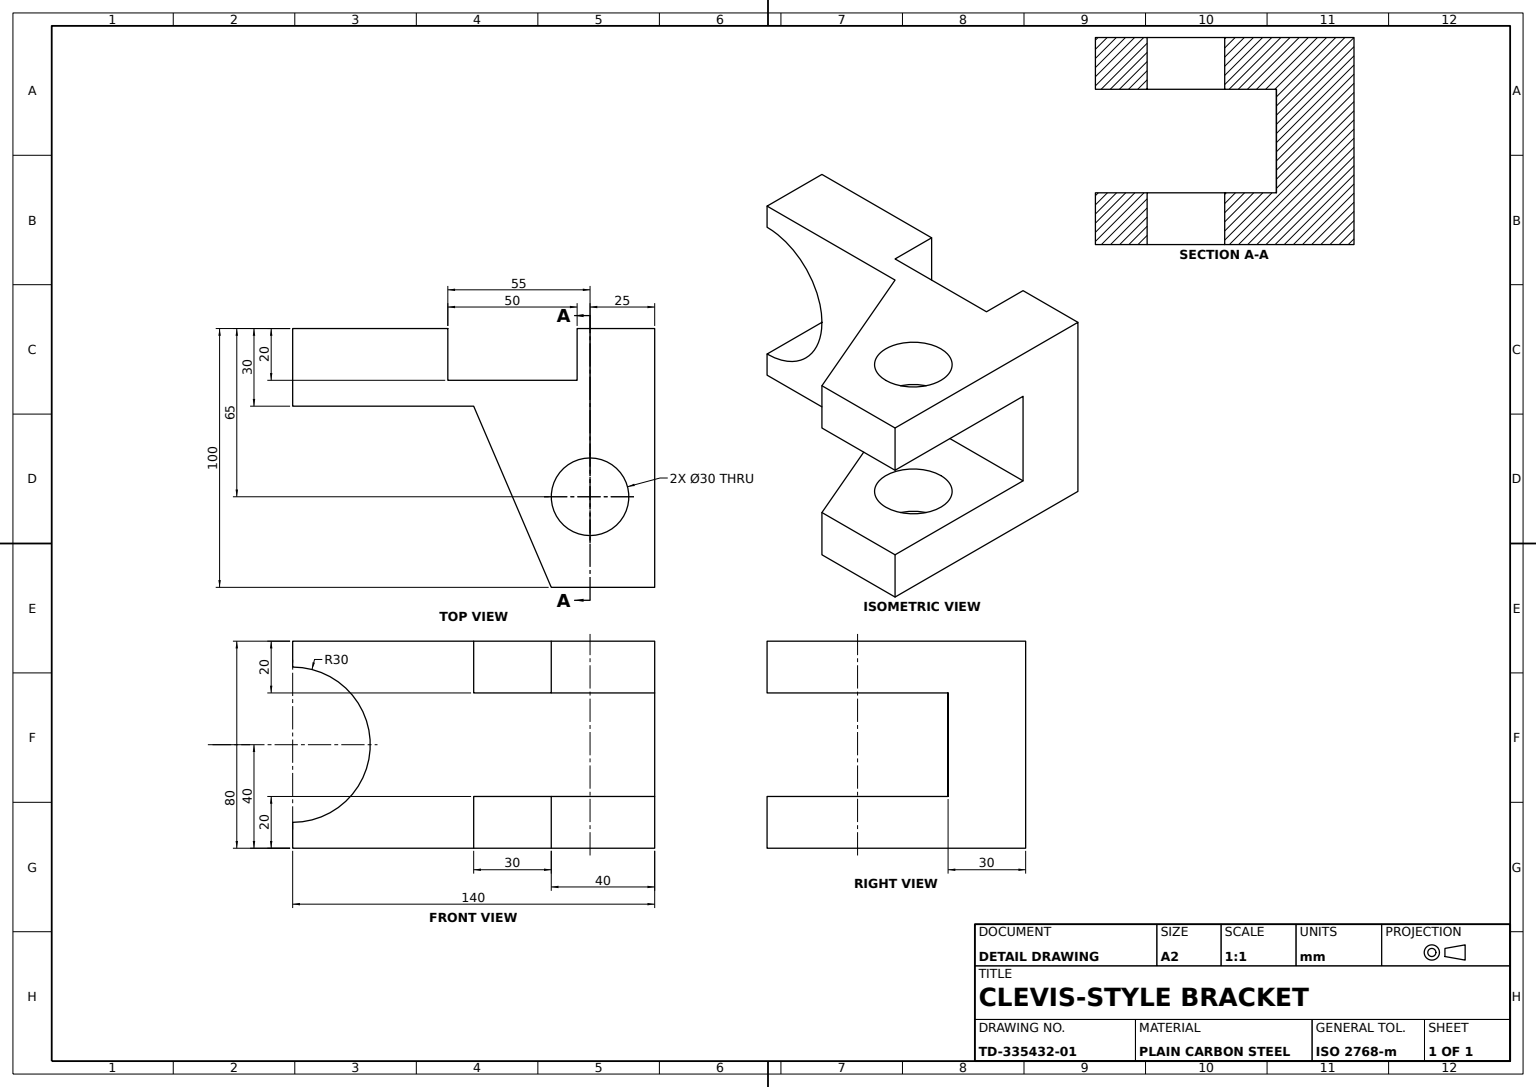
from build123d import *

# Parameters (mm, degrees)
BASE_BLOCK_DEPTH           = 30
SIDE_BOSS_DEPTH            = 20
TOP_BOSS_DEPTH             = 20
THROUGH_HOLE_SKETCH_R      = 15
COAXIAL_THROUGH_HOLE_DEPTH = 80
CURVED_RELIEF_SKETCH_W     = 50
CURVED_RELIEF_SKETCH_H     = 20
CURVED_RELIEF_CUT_DEPTH    = 80


with BuildPart() as part:
    # Base Profile Sketch → Base Block (new body)
    with BuildSketch(Plane.XY):
        with BuildLine():
            Line((140, 0), (0, 0))
            Line((0, 0), (0, -10))
            ThreePointArc((0, -10), (30, -40), (0, -70))
            Line((0, -70), (0, -80))
            Line((0, -80), (140, -80))
            Line((140, -80), (140, 0))
        make_face()
    extrude(amount=BASE_BLOCK_DEPTH)

    # Side Boss Sketch → Side Boss (add)
    with BuildSketch(Plane.XZ.offset(80)):
        Polygon((140, 30), (140, 100), (100, 100), (70, 30), align=None)
    extrude(amount=-SIDE_BOSS_DEPTH)

    # Top Boss Sketch → Top Boss (add)
    with BuildSketch(Plane(origin=(0, 0, 0), x_dir=(1, 0, 0), z_dir=(0, 1, 0))):
        Polygon((140, -30), (140, -100), (100, -100), (70, -30), align=None)
    extrude(amount=-TOP_BOSS_DEPTH)

    # Through Hole Sketch → Coaxial Through Hole (cut)
    with BuildSketch(Plane.XZ.offset(80)):
        with Locations(Location((115, 65, 0), (0, 0, 270))):
            Circle(THROUGH_HOLE_SKETCH_R)
    extrude(amount=-COAXIAL_THROUGH_HOLE_DEPTH, mode=Mode.SUBTRACT)

    # Curved Relief Sketch → Curved Relief Cut (cut)
    with BuildSketch(Plane.XZ.offset(80)):
        with Locations((85, 10)):
            Rectangle(CURVED_RELIEF_SKETCH_W, CURVED_RELIEF_SKETCH_H)
    extrude(amount=-CURVED_RELIEF_CUT_DEPTH, mode=Mode.SUBTRACT)


solid = part.part
